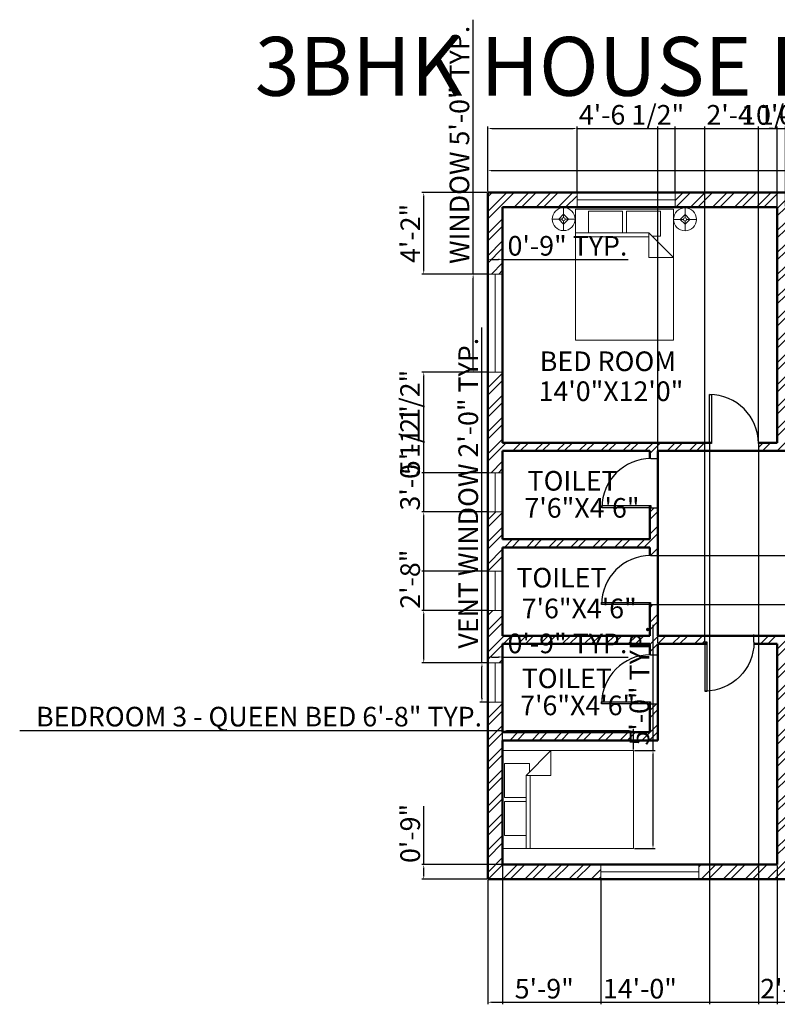
# Model space of a CAD drawing. Units: inches. Extents: x 1954 to 2815, y 1733 to 2371.
# Tile 1 of 4: x 1954 to 2417, y 1769 to 2371. Entities that reach past the tile are written whole.
import ezdxf

# ---------------------------------------------------------------- set-up
doc = ezdxf.new("R2010")
doc.units = ezdxf.units.IN
for name, color, linetype, lineweight in [('A-ANNO-DIMS', 2, 'Continuous', 18), ('A-ANNO-TEXT', 7, 'Continuous', 25), ('A-AREA-IDEN', 7, 'Continuous', 25), ('A-DOOR', 3, 'Continuous', 25), ('A-FURN', 8, 'Continuous', 18), ('A-GLAZ', 4, 'Continuous', 18), ('A-WALL', 7, 'Continuous', 50), ('A-WALL-PATT', 252, 'Continuous', 13)]:
    doc.layers.add(name, color=color, linetype=linetype, lineweight=lineweight)
doc.styles.get("Standard").update_dxf_attribs({"font": 'arial.ttf'})
doc.dimstyles.new('ISO-25', dxfattribs={"dimtxt": 12, "dimasz": 2.5, "dimexe": 1.25, "dimexo": 0.625, "dimtad": 1, "dimdec": 1, "dimlunit": 4, "dimtxsty": 'Standard', "dimcen": 2.5, "dimadec": 0, "dimazin": 0, "dimtfac": 1, "dimtdec": 1, "dimtmove": 0, "dimatfit": 3, "dimfxl": 1, "dimarcsym": 0})

# ---------------------------------------------------------------- blocks, each defined once
blk = doc.blocks.new('*U2')
for p, q in [((0, 0), (0, -6)), ((40, 0), (40, -6))]:
    blk.add_line(p, q)
blk.add_lwpolyline([(0, 0), (0, 40), (1.75, 40), (1.75, 0)], close=True)
blk.add_arc((0, 0), 40, 0, 90)
blk = doc.blocks.new('Bed - Queen')
for p, q in [((0, -80.00003), (0, 0)), ((0, 0), (59.99999, 0)), ((59.99999, 0), (59.99999, -80.00003)), ((7.99999, -1.2), (28.79998, -1.2)), ((7.99999, -14.4), (7.99999, -1.2)), ((28.79998, -1.2), (28.79998, -14.4)), ((31.19999, -1.2), (51.99999, -1.2)), ((31.19999, -14.4), (31.19999, -1.2)), ((51.99999, -1.2), (51.99999, -16.4)), ((0, -14.4), (44.8, -14.4)), ((44.8, -16.8), (0, -16.8)), ((59.99999, -29.6), (44.8, -14.4)), ((44.8, -14.4), (44.8, -29.6)), ((51.99999, -16.4), (46.79936, -16.4)), ((44.8, -29.6), (59.99999, -29.6)), ((59.99999, -80.00003), (0, -80.00003))]:
    blk.add_line(p, q)
blk = doc.blocks.new('Lamp - Table')
for p, q in [((0, 7), (0, 1)), ((-1, 0), (-7, 0)), ((0, 3), (-3, 0)), ((-3, 0), (0, -3)), ((3, 0), (0, 3)), ((0, -3), (3, 0)), ((1, 0), (7, 0)), ((0, -1), (0, -7))]:
    blk.add_line(p, q)
for radius in [7, 1]:
    blk.add_circle((0, 0), radius)
blk = doc.blocks.new('*D10')
at = {"layer": 'A-ANNO-DIMS', "color": 0, "lineweight": -2, "transparency": 16777216}
for p, q in [((2239.88, 2265.61), (2239.88, 2279.68)), ((2242.38, 2278.43), (2717.38, 2278.43)), ((2719.88, 2265.61), (2719.88, 2279.68))]:
    blk.add_line(p, q, dxfattribs=at)
at = {"layer": 'A-ANNO-DIMS', "color": 0, "transparency": 16777216}
for points in [[(2242.38, 2278.85), (2242.38, 2278.01), (2239.88, 2278.43)], [(2717.38, 2278.85), (2717.38, 2278.01), (2719.88, 2278.43)]]:
    blk.add_solid(points, dxfattribs=at)
at = {"layer": 'Defpoints', "color": 0, "transparency": 16777216}
for p in [(2719.88, 2278.43), (2239.88, 2264.98), (2719.88, 2264.98)]:
    blk.add_point(p, dxfattribs=at)
at = {"layer": 'A-ANNO-DIMS', "color": 0, "transparency": 16777216, "insert": (2479.88, 2285.18), "char_height": 12, "attachment_point": 5}
blk.add_mtext("40'", dxfattribs=at)
blk = doc.blocks.new('WIN-60IN')
blk.add_line((4.5, 60), (4.5, 0))
blk.add_lwpolyline([(9, 60), (9, 0), (0, 0), (0, 60)], close=True)
blk = doc.blocks.new('VENT-WIN-24IN')
blk.add_line((4.5, 24), (4.5, 0))
blk.add_lwpolyline([(9, 24), (9, 0), (0, 0), (0, 24)], close=True)
blk = doc.blocks.new('*D14')
at = {"layer": 'A-ANNO-DIMS', "color": 0, "lineweight": -2, "transparency": 16777216}
for p, q in [((2230.88, 2215.14), (2230.88, 2370.74)), ((2239.26, 2215.14), (2229.63, 2215.14)), ((2230.88, 2157.64), (2230.88, 2212.64)), ((2239.26, 2155.14), (2229.63, 2155.14))]:
    blk.add_line(p, q, dxfattribs=at)
at = {"layer": 'A-ANNO-DIMS', "color": 0, "transparency": 16777216}
for points in [[(2230.47, 2212.64), (2231.3, 2212.64), (2230.88, 2215.14)], [(2230.47, 2157.64), (2231.3, 2157.64), (2230.88, 2155.14)]]:
    blk.add_solid(points, dxfattribs=at)
at = {"layer": 'Defpoints', "color": 0, "transparency": 16777216}
for p in [(2230.88, 2215.14), (2239.88, 2215.14), (2239.88, 2155.14)]:
    blk.add_point(p, dxfattribs=at)
at = {"layer": 'A-ANNO-DIMS', "color": 0, "transparency": 16777216, "insert": (2224.05, 2294.19), "char_height": 12, "attachment_point": 5, "rotation": 90}
blk.add_mtext('WINDOW 5\'-0" TYP.', dxfattribs=at)
blk = doc.blocks.new('*D15')
at = {"layer": 'A-ANNO-DIMS', "color": 0, "lineweight": -2, "transparency": 16777216}
for p, q in [((2239.88, 2215.77), (2239.88, 2225.39)), ((2242.38, 2224.14), (2246.38, 2224.14)), ((2248.88, 2215.77), (2248.88, 2225.39)), ((2248.88, 2224.14), (2325.78, 2224.14))]:
    blk.add_line(p, q, dxfattribs=at)
at = {"layer": 'A-ANNO-DIMS', "color": 0, "transparency": 16777216}
for points in [[(2242.38, 2224.56), (2242.38, 2223.73), (2239.88, 2224.14)], [(2246.38, 2224.56), (2246.38, 2223.73), (2248.88, 2224.14)]]:
    blk.add_solid(points, dxfattribs=at)
at = {"layer": 'Defpoints', "color": 0, "transparency": 16777216}
for p in [(2248.88, 2224.14), (2239.88, 2215.14), (2248.88, 2215.14)]:
    blk.add_point(p, dxfattribs=at)
at = {"layer": 'A-ANNO-DIMS', "color": 0, "transparency": 16777216, "insert": (2288.58, 2230.89), "char_height": 12, "attachment_point": 5}
blk.add_mtext('0\'-9" TYP.', dxfattribs=at)
blk = doc.blocks.new('*D18')
at = {"layer": 'A-ANNO-DIMS', "color": 0, "lineweight": -2, "transparency": 16777216}
for p, q in [((2248.88, 1935.73), (1953.62, 1935.73)), ((2248.88, 1924.36), (2248.88, 1936.98)), ((2326.38, 1935.73), (2251.38, 1935.73)), ((2328.88, 1924.36), (2328.88, 1936.98))]:
    blk.add_line(p, q, dxfattribs=at)
at = {"layer": 'A-ANNO-DIMS', "color": 0, "transparency": 16777216}
for points in [[(2251.38, 1936.15), (2251.38, 1935.32), (2248.88, 1935.73)], [(2326.38, 1936.15), (2326.38, 1935.32), (2328.88, 1935.73)]]:
    blk.add_solid(points, dxfattribs=at)
at = {"layer": 'Defpoints', "color": 0, "transparency": 16777216}
for p in [(2248.88, 1935.73), (2248.88, 1923.73), (2328.88, 1923.73)]:
    blk.add_point(p, dxfattribs=at)
at = {"layer": 'A-ANNO-DIMS', "color": 0, "transparency": 16777216, "insert": (2100, 1942.93), "char_height": 12, "attachment_point": 5}
blk.add_mtext('BEDROOM 3 - QUEEN BED 6\'-8" TYP.', dxfattribs=at)
blk = doc.blocks.new('*D19')
at = {"layer": 'A-ANNO-DIMS', "color": 0, "lineweight": -2, "transparency": 16777216}
for p, q in [((2340.88, 1923.73), (2340.88, 2000.63)), ((2329.51, 1923.73), (2342.13, 1923.73)), ((2340.88, 1866.23), (2340.88, 1921.23)), ((2329.51, 1863.73), (2342.13, 1863.73))]:
    blk.add_line(p, q, dxfattribs=at)
at = {"layer": 'A-ANNO-DIMS', "color": 0, "transparency": 16777216}
for points in [[(2340.47, 1921.23), (2341.3, 1921.23), (2340.88, 1923.73)], [(2340.47, 1866.23), (2341.3, 1866.23), (2340.88, 1863.73)]]:
    blk.add_solid(points, dxfattribs=at)
at = {"layer": 'Defpoints', "color": 0, "transparency": 16777216}
for p in [(2328.88, 1923.73), (2340.88, 1923.73), (2328.88, 1863.73)]:
    blk.add_point(p, dxfattribs=at)
at = {"layer": 'A-ANNO-DIMS', "color": 0, "transparency": 16777216, "insert": (2334.13, 1963.43), "char_height": 12, "attachment_point": 5, "rotation": 90}
blk.add_mtext('5\'-0" TYP.', dxfattribs=at)
blk = doc.blocks.new('*D20')
at = {"layer": 'A-ANNO-DIMS', "color": 0, "lineweight": -2, "transparency": 16777216}
for p, q in [((2236.28, 1977.35), (2236.28, 2182.45)), ((2239.26, 1977.35), (2235.03, 1977.35)), ((2236.28, 1955.85), (2236.28, 1974.85)), ((2239.26, 1953.35), (2235.03, 1953.35))]:
    blk.add_line(p, q, dxfattribs=at)
at = {"layer": 'A-ANNO-DIMS', "color": 0, "transparency": 16777216}
for points in [[(2235.87, 1974.85), (2236.7, 1974.85), (2236.28, 1977.35)], [(2235.87, 1955.85), (2236.7, 1955.85), (2236.28, 1953.35)]]:
    blk.add_solid(points, dxfattribs=at)
at = {"layer": 'Defpoints', "color": 0, "transparency": 16777216}
for p in [(2236.28, 1977.35), (2239.88, 1977.35), (2239.88, 1953.35)]:
    blk.add_point(p, dxfattribs=at)
at = {"layer": 'A-ANNO-DIMS', "color": 0, "transparency": 16777216, "insert": (2229.45, 2081.15), "char_height": 12, "attachment_point": 5, "rotation": 90}
blk.add_mtext('VENT WINDOW 2\'-0" TYP.', dxfattribs=at)
blk = doc.blocks.new('*D21')
at = {"layer": 'A-ANNO-DIMS', "color": 0, "lineweight": -2, "transparency": 16777216}
for p, q in [((2239.88, 1977.98), (2239.88, 1982.2)), ((2248.88, 1977.98), (2248.88, 1982.2)), ((2242.38, 1980.95), (2246.38, 1980.95)), ((2248.88, 1980.95), (2325.78, 1980.95))]:
    blk.add_line(p, q, dxfattribs=at)
at = {"layer": 'A-ANNO-DIMS', "color": 0, "transparency": 16777216}
for points in [[(2242.38, 1981.37), (2242.38, 1980.54), (2239.88, 1980.95)], [(2246.38, 1981.37), (2246.38, 1980.54), (2248.88, 1980.95)]]:
    blk.add_solid(points, dxfattribs=at)
at = {"layer": 'Defpoints', "color": 0, "transparency": 16777216}
for p in [(2239.88, 1977.35), (2248.88, 1980.95), (2248.88, 1977.35)]:
    blk.add_point(p, dxfattribs=at)
at = {"layer": 'A-ANNO-DIMS', "color": 0, "transparency": 16777216, "insert": (2288.58, 1987.71), "char_height": 12, "attachment_point": 5}
blk.add_mtext('0\'-9" TYP.', dxfattribs=at)
blk = doc.blocks.new('*D30')
at = {"layer": 'A-ANNO-DIMS', "color": 0, "lineweight": -2, "transparency": 16777216}
for p, q in [((2248.88, 1853.36), (2248.88, 1768.53)), ((2416.88, 1853.36), (2416.88, 1768.53)), ((2251.38, 1769.78), (2414.38, 1769.78))]:
    blk.add_line(p, q, dxfattribs=at)
at = {"layer": 'A-ANNO-DIMS', "color": 0, "transparency": 16777216}
for points in [[(2251.38, 1770.2), (2251.38, 1769.37), (2248.88, 1769.78)], [(2414.38, 1770.2), (2414.38, 1769.37), (2416.88, 1769.78)]]:
    blk.add_solid(points, dxfattribs=at)
at = {"layer": 'Defpoints', "color": 0, "transparency": 16777216}
for p in [(2248.88, 1853.98), (2416.88, 1853.98), (2416.88, 1769.78)]:
    blk.add_point(p, dxfattribs=at)
at = {"layer": 'A-ANNO-DIMS', "color": 0, "transparency": 16777216, "insert": (2332.88, 1776.53), "char_height": 12, "attachment_point": 5}
blk.add_mtext('14\'-0"', dxfattribs=at)
blk = doc.blocks.new('*D36')
at = {"layer": 'A-ANNO-DIMS', "color": 0, "lineweight": -2, "transparency": 16777216}
for p, q in [((2200.68, 1853.98), (2200.68, 1889.63)), ((2248.26, 1853.98), (2199.43, 1853.98)), ((2200.68, 1847.48), (2200.68, 1851.48)), ((2239.26, 1844.98), (2199.43, 1844.98))]:
    blk.add_line(p, q, dxfattribs=at)
at = {"layer": 'A-ANNO-DIMS', "color": 0, "transparency": 16777216}
for points in [[(2200.27, 1851.48), (2201.1, 1851.48), (2200.68, 1853.98)], [(2200.27, 1847.48), (2201.1, 1847.48), (2200.68, 1844.98)]]:
    blk.add_solid(points, dxfattribs=at)
at = {"layer": 'Defpoints', "color": 0, "transparency": 16777216}
for p in [(2200.68, 1853.98), (2248.88, 1853.98), (2239.88, 1844.98)]:
    blk.add_point(p, dxfattribs=at)
at = {"layer": 'A-ANNO-DIMS', "color": 0, "transparency": 16777216, "insert": (2193.93, 1873.06), "char_height": 12, "attachment_point": 5, "rotation": 90}
blk.add_mtext('0\'-9"', dxfattribs=at)
blk = doc.blocks.new('*D37')
at = {"layer": 'A-ANNO-DIMS', "color": 0, "lineweight": -2, "transparency": 16777216}
for p, q in [((2414.38, 2304.18), (2411.88, 2304.18)), ((2416.88, 2256.61), (2416.88, 2305.43)), ((2416.88, 2304.18), (2421.88, 2304.18)), ((2421.88, 2256.61), (2421.88, 2305.43)), ((2424.38, 2304.18), (2460.03, 2304.18))]:
    blk.add_line(p, q, dxfattribs=at)
at = {"layer": 'A-ANNO-DIMS', "color": 0, "transparency": 16777216}
for points in [[(2414.38, 2304.6), (2414.38, 2303.77), (2416.88, 2304.18)], [(2424.38, 2304.6), (2424.38, 2303.77), (2421.88, 2304.18)]]:
    blk.add_solid(points, dxfattribs=at)
at = {"layer": 'Defpoints', "color": 0, "transparency": 16777216}
for p in [(2421.88, 2304.18), (2416.88, 2255.98), (2421.88, 2255.98)]:
    blk.add_point(p, dxfattribs=at)
at = {"layer": 'A-ANNO-DIMS', "color": 0, "transparency": 16777216, "insert": (2443.46, 2310.93), "char_height": 12, "attachment_point": 5}
blk.add_mtext('0\'-5"', dxfattribs=at)
blk = doc.blocks.new('*D38')
at = {"layer": 'A-ANNO-DIMS', "color": 0, "lineweight": -2, "transparency": 16777216}
for p, q in [((2239.88, 2265.61), (2239.88, 2305.43)), ((2242.38, 2304.18), (2291.96, 2304.18)), ((2294.46, 2265.61), (2294.46, 2305.43)), ((2294.46, 2304.18), (2358.55, 2304.18))]:
    blk.add_line(p, q, dxfattribs=at)
at = {"layer": 'A-ANNO-DIMS', "color": 0, "transparency": 16777216}
for points in [[(2242.38, 2304.6), (2242.38, 2303.77), (2239.88, 2304.18)], [(2291.96, 2304.6), (2291.96, 2303.77), (2294.46, 2304.18)]]:
    blk.add_solid(points, dxfattribs=at)
at = {"layer": 'Defpoints', "color": 0, "transparency": 16777216}
for p in [(2294.46, 2304.18), (2239.88, 2264.98), (2294.46, 2264.98)]:
    blk.add_point(p, dxfattribs=at)
at = {"layer": 'A-ANNO-DIMS', "color": 0, "transparency": 16777216, "insert": (2327.76, 2311.01), "char_height": 12, "attachment_point": 5}
blk.add_mtext('4\'-6 1/2"', dxfattribs=at)
blk = doc.blocks.new('*D39')
at = {"layer": 'A-ANNO-DIMS', "color": 0, "lineweight": -2, "transparency": 16777216}
for p, q in [((2354.46, 2265.61), (2354.46, 2305.43)), ((2356.96, 2304.18), (2477.93, 2304.18)), ((2480.43, 2265.61), (2480.43, 2305.43))]:
    blk.add_line(p, q, dxfattribs=at)
at = {"layer": 'A-ANNO-DIMS', "color": 0, "transparency": 16777216}
for points in [[(2356.96, 2304.6), (2356.96, 2303.77), (2354.46, 2304.18)], [(2477.93, 2304.6), (2477.93, 2303.77), (2480.43, 2304.18)]]:
    blk.add_solid(points, dxfattribs=at)
at = {"layer": 'Defpoints', "color": 0, "transparency": 16777216}
for p in [(2480.43, 2304.18), (2354.46, 2264.98), (2480.43, 2264.98)]:
    blk.add_point(p, dxfattribs=at)
at = {"layer": 'A-ANNO-DIMS', "color": 0, "transparency": 16777216, "insert": (2417.44, 2310.93), "char_height": 12, "attachment_point": 5}
blk.add_mtext('10\'-6"', dxfattribs=at)
blk = doc.blocks.new('*D40')
at = {"layer": 'A-ANNO-DIMS', "color": 0, "lineweight": -2, "transparency": 16777216}
for p, q in [((2239.88, 1844.36), (2239.88, 1768.53)), ((2308.9, 1844.36), (2308.9, 1768.53)), ((2242.38, 1769.78), (2306.4, 1769.78))]:
    blk.add_line(p, q, dxfattribs=at)
at = {"layer": 'A-ANNO-DIMS', "color": 0, "transparency": 16777216}
for points in [[(2242.38, 1770.2), (2242.38, 1769.37), (2239.88, 1769.78)], [(2306.4, 1770.2), (2306.4, 1769.37), (2308.9, 1769.78)]]:
    blk.add_solid(points, dxfattribs=at)
at = {"layer": 'Defpoints', "color": 0, "transparency": 16777216}
for p in [(2239.88, 1844.98), (2308.9, 1844.98), (2308.9, 1769.78)]:
    blk.add_point(p, dxfattribs=at)
at = {"layer": 'A-ANNO-DIMS', "color": 0, "transparency": 16777216, "insert": (2274.39, 1776.53), "char_height": 12, "attachment_point": 5}
blk.add_mtext('5\'-9"', dxfattribs=at)
blk = doc.blocks.new('*D41')
at = {"layer": 'A-ANNO-DIMS', "color": 0, "lineweight": -2, "transparency": 16777216}
for p, q in [((2239.26, 2264.98), (2199.43, 2264.98)), ((2200.68, 2217.64), (2200.68, 2262.48)), ((2239.26, 2215.14), (2199.43, 2215.14))]:
    blk.add_line(p, q, dxfattribs=at)
at = {"layer": 'A-ANNO-DIMS', "color": 0, "transparency": 16777216}
for points in [[(2200.27, 2262.48), (2201.1, 2262.48), (2200.68, 2264.98)], [(2200.27, 2217.64), (2201.1, 2217.64), (2200.68, 2215.14)]]:
    blk.add_solid(points, dxfattribs=at)
at = {"layer": 'Defpoints', "color": 0, "transparency": 16777216}
for p in [(2200.68, 2264.98), (2239.88, 2264.98), (2239.88, 2215.14)]:
    blk.add_point(p, dxfattribs=at)
at = {"layer": 'A-ANNO-DIMS', "color": 0, "transparency": 16777216, "insert": (2194.03, 2240.06), "char_height": 12, "attachment_point": 5, "rotation": 90}
blk.add_mtext('4\'-2"', dxfattribs=at)
blk = doc.blocks.new('*D42')
at = {"layer": 'A-ANNO-DIMS', "color": 0, "lineweight": -2, "transparency": 16777216}
for p, q in [((2239.26, 2155.14), (2199.43, 2155.14)), ((2200.68, 2096.18), (2200.68, 2152.64)), ((2239.26, 2093.68), (2199.43, 2093.68))]:
    blk.add_line(p, q, dxfattribs=at)
at = {"layer": 'A-ANNO-DIMS', "color": 0, "transparency": 16777216}
for points in [[(2200.27, 2152.64), (2201.1, 2152.64), (2200.68, 2155.14)], [(2200.27, 2096.18), (2201.1, 2096.18), (2200.68, 2093.68)]]:
    blk.add_solid(points, dxfattribs=at)
at = {"layer": 'Defpoints', "color": 0, "transparency": 16777216}
for p in [(2200.68, 2155.14), (2239.88, 2155.14), (2239.88, 2093.68)]:
    blk.add_point(p, dxfattribs=at)
at = {"layer": 'A-ANNO-DIMS', "color": 0, "transparency": 16777216, "insert": (2193.85, 2124.41), "char_height": 12, "attachment_point": 5, "rotation": 90}
blk.add_mtext('5\'-1 1/2"', dxfattribs=at)
blk = doc.blocks.new('*D43')
at = {"layer": 'A-ANNO-DIMS', "color": 0, "lineweight": -2, "transparency": 16777216}
for p, q in [((2200.68, 2069.68), (2200.68, 2133.29)), ((2239.26, 2069.68), (2199.43, 2069.68)), ((2200.68, 2035.9), (2200.68, 2067.18)), ((2239.26, 2033.4), (2199.43, 2033.4))]:
    blk.add_line(p, q, dxfattribs=at)
at = {"layer": 'A-ANNO-DIMS', "color": 0, "transparency": 16777216}
for points in [[(2200.27, 2067.18), (2201.1, 2067.18), (2200.68, 2069.68)], [(2200.27, 2035.9), (2201.1, 2035.9), (2200.68, 2033.4)]]:
    blk.add_solid(points, dxfattribs=at)
at = {"layer": 'Defpoints', "color": 0, "transparency": 16777216}
for p in [(2200.68, 2069.68), (2239.88, 2069.68), (2239.88, 2033.4)]:
    blk.add_point(p, dxfattribs=at)
at = {"layer": 'A-ANNO-DIMS', "color": 0, "transparency": 16777216, "insert": (2193.85, 2102.74), "char_height": 12, "attachment_point": 5, "rotation": 90}
blk.add_mtext('3\'-0 1/2"', dxfattribs=at)
blk = doc.blocks.new('*D44')
at = {"layer": 'A-ANNO-DIMS', "color": 0, "lineweight": -2, "transparency": 16777216}
for p, q in [((2200.68, 2009.4), (2200.68, 2045.25)), ((2239.26, 2009.4), (2199.43, 2009.4)), ((2200.68, 1979.85), (2200.68, 2006.9)), ((2239.26, 1977.35), (2199.43, 1977.35))]:
    blk.add_line(p, q, dxfattribs=at)
at = {"layer": 'A-ANNO-DIMS', "color": 0, "transparency": 16777216}
for points in [[(2200.27, 2006.9), (2201.1, 2006.9), (2200.68, 2009.4)], [(2200.27, 1979.85), (2201.1, 1979.85), (2200.68, 1977.35)]]:
    blk.add_solid(points, dxfattribs=at)
at = {"layer": 'Defpoints', "color": 0, "transparency": 16777216}
for p in [(2200.68, 2009.4), (2239.88, 2009.4), (2239.88, 1977.35)]:
    blk.add_point(p, dxfattribs=at)
at = {"layer": 'A-ANNO-DIMS', "color": 0, "transparency": 16777216, "insert": (2193.93, 2028.57), "char_height": 12, "attachment_point": 5, "rotation": 90}
blk.add_mtext('2\'-8"', dxfattribs=at)
blk = doc.blocks.new('*D47')
at = {"layer": 'A-ANNO-DIMS', "color": 0, "lineweight": -2, "transparency": 16777216}
for p, q in [((2375.36, 2106.36), (2375.36, 1768.53)), ((2405.36, 2106.36), (2405.36, 1768.53)), ((2377.86, 1769.78), (2402.86, 1769.78)), ((2405.36, 1769.78), (2441.21, 1769.78))]:
    blk.add_line(p, q, dxfattribs=at)
at = {"layer": 'A-ANNO-DIMS', "color": 0, "transparency": 16777216}
for points in [[(2377.86, 1770.2), (2377.86, 1769.37), (2375.36, 1769.78)], [(2402.86, 1770.2), (2402.86, 1769.37), (2405.36, 1769.78)]]:
    blk.add_solid(points, dxfattribs=at)
at = {"layer": 'Defpoints', "color": 0, "transparency": 16777216}
for p in [(2375.36, 2106.98), (2405.36, 2106.98), (2405.36, 1769.78)]:
    blk.add_point(p, dxfattribs=at)
at = {"layer": 'A-ANNO-DIMS', "color": 0, "transparency": 16777216, "insert": (2424.53, 1776.53), "char_height": 12, "attachment_point": 5}
blk.add_mtext('2\'-6"', dxfattribs=at)
blk = doc.blocks.new('*D48')
at = {"layer": 'A-ANNO-DIMS', "color": 0, "lineweight": -2, "transparency": 16777216}
for p, q in [((2405.35, 2112.61), (2405.35, 2305.43)), ((2407.85, 2304.18), (2414.38, 2304.18)), ((2416.88, 2112.61), (2416.88, 2305.43)), ((2416.88, 2304.18), (2489.82, 2304.18))]:
    blk.add_line(p, q, dxfattribs=at)
at = {"layer": 'A-ANNO-DIMS', "color": 0, "transparency": 16777216}
for points in [[(2407.85, 2304.6), (2407.85, 2303.77), (2405.35, 2304.18)], [(2414.38, 2304.6), (2414.38, 2303.77), (2416.88, 2304.18)]]:
    blk.add_solid(points, dxfattribs=at)
at = {"layer": 'Defpoints', "color": 0, "transparency": 16777216}
for p in [(2416.88, 2304.18), (2405.35, 2111.98), (2416.88, 2111.98)]:
    blk.add_point(p, dxfattribs=at)
at = {"layer": 'A-ANNO-DIMS', "color": 0, "transparency": 16777216, "insert": (2454.6, 2311.01), "char_height": 12, "attachment_point": 5}
blk.add_mtext('0\'-11 1/2"', dxfattribs=at)
blk = doc.blocks.new('*D52')
at = {"layer": 'A-ANNO-DIMS', "color": 0, "lineweight": -2, "transparency": 16777216}
for p, q in [((2759.08, 2043), (2759.08, 2078.85)), ((2344.56, 2043), (2760.33, 2043)), ((2759.08, 2015.5), (2759.08, 2040.5)), ((2344.56, 2013), (2760.33, 2013))]:
    blk.add_line(p, q, dxfattribs=at)
at = {"layer": 'A-ANNO-DIMS', "color": 0, "transparency": 16777216}
for points in [[(2758.67, 2040.5), (2759.5, 2040.5), (2759.08, 2043)], [(2758.67, 2015.5), (2759.5, 2015.5), (2759.08, 2013)]]:
    blk.add_solid(points, dxfattribs=at)
at = {"layer": 'Defpoints', "color": 0, "transparency": 16777216}
for p in [(2343.94, 2043), (2759.08, 2043), (2343.94, 2013)]:
    blk.add_point(p, dxfattribs=at)
at = {"layer": 'A-ANNO-DIMS', "color": 0, "transparency": 16777216, "insert": (2752.33, 2062.18), "char_height": 12, "attachment_point": 5, "rotation": 90}
blk.add_mtext('2\'-6"', dxfattribs=at)
blk = doc.blocks.new('*D55')
at = {"layer": 'A-ANNO-DIMS', "color": 0, "lineweight": -2, "transparency": 16777216}
for p, q in [((2343.88, 1989.61), (2343.88, 2305.43)), ((2346.38, 2304.18), (2370.09, 2304.18)), ((2372.59, 1990.74), (2372.59, 2305.43)), ((2372.59, 2304.18), (2436.4, 2304.18))]:
    blk.add_line(p, q, dxfattribs=at)
at = {"layer": 'A-ANNO-DIMS', "color": 0, "transparency": 16777216}
for points in [[(2346.38, 2304.6), (2346.38, 2303.77), (2343.88, 2304.18)], [(2370.09, 2304.6), (2370.09, 2303.77), (2372.59, 2304.18)]]:
    blk.add_solid(points, dxfattribs=at)
at = {"layer": 'Defpoints', "color": 0, "transparency": 16777216}
for p in [(2372.59, 2304.18), (2343.88, 1988.98), (2372.59, 1990.12)]:
    blk.add_point(p, dxfattribs=at)
at = {"layer": 'A-ANNO-DIMS', "color": 0, "transparency": 16777216, "insert": (2405.75, 2311.01), "char_height": 12, "attachment_point": 5}
blk.add_mtext('2\'-4 1/2"', dxfattribs=at)

msp = doc.modelspace()

# ---------------------------------------------------------------- hatches: boundary and pattern name
at = {"layer": 'A-WALL-PATT'}
h = msp.add_hatch(dxfattribs=at)
h.set_pattern_fill('ANSI32', color=256)
h.paths.add_polyline_path([(2294.46, 2264.98), (2239.88, 2264.98), (2239.88, 2215.14), (2248.88, 2215.14), (2248.88, 2255.98), (2294.46, 2255.98)])
h = msp.add_hatch(dxfattribs=at)
h.set_pattern_fill('ANSI32', color=256)
h.paths.add_polyline_path([(2480.43, 2264.98), (2354.46, 2264.98), (2354.46, 2255.98), (2416.88, 2255.98), (2416.88, 2111.98), (2405.35, 2111.98, -0.004167), (2405.36, 2111.48), (2405.36, 2106.98), (2487.77, 2106.98), (2487.77, 2111.48), (2487.77, 2111.98), (2421.88, 2111.98), (2421.88, 2255.98), (2480.43, 2255.98)])
h.paths.add_polyline_path([(2719.88, 2264.98), (2540.43, 2264.98), (2540.43, 2255.98), (2589.88, 2255.98), (2589.88, 2111.98), (2517.77, 2111.98, -0.004167), (2517.77, 2111.48), (2517.77, 2106.98), (2631.3, 2106.98), (2631.3, 2111.98), (2594.88, 2111.98), (2594.88, 2255.98), (2710.88, 2255.98), (2710.88, 2213), (2719.88, 2213)])
h = msp.add_hatch(dxfattribs=at)
h.set_pattern_fill('ANSI32', color=256)
h.paths.add_polyline_path([(2375.36, 2111.48), (2375.36, 2111.98), (2248.88, 2111.98), (2248.88, 2155.14), (2239.88, 2155.14), (2239.88, 2093.68), (2248.88, 2093.68), (2248.88, 2106.98), (2338.88, 2106.98), (2338.88, 2102.27, -0.006284), (2339.64, 2102.28), (2343.88, 2102.28), (2343.88, 2106.98), (2375.36, 2106.98)])
h.paths.add_polyline_path([(2343.88, 2052.98), (2343.88, 2072.28), (2339.64, 2072.28), (2338.88, 2072.28), (2338.88, 2052.98), (2248.88, 2052.98), (2248.88, 2069.68), (2239.88, 2069.68), (2239.88, 2033.4), (2248.88, 2033.4), (2248.88, 2047.98), (2338.88, 2047.98), (2338.88, 2042.99, -0.004601), (2339.44, 2043), (2343.88, 2043)])
h = msp.add_hatch(dxfattribs=at)
h.set_pattern_fill('ANSI32', color=256)
h.paths.add_polyline_path([(2372.59, 1993.98), (2343.88, 1993.98), (2343.88, 2013), (2339.44, 2013), (2338.88, 2013), (2338.88, 1993.98), (2248.88, 1993.98), (2248.88, 2009.4), (2239.88, 2009.4), (2239.88, 1977.35), (2248.88, 1977.35), (2248.88, 1988.98), (2338.88, 1988.98), (2338.88, 1982.3, -0.004167), (2339.38, 1982.31), (2343.88, 1982.31), (2343.88, 1988.98), (2372.59, 1988.98), (2372.59, 1990.12)])
h = msp.add_hatch(dxfattribs=at)
h.set_pattern_fill('ANSI32', color=256)
h.paths.add_polyline_path([(2585.41, 1844.98), (2585.41, 1849.48, -0.03766), (2585.75, 1853.98), (2486.88, 1853.98), (2486.88, 1942.98), (2471.49, 1942.98), (2471.49, 1937.98), (2481.88, 1937.98), (2481.88, 1853.98), (2421.88, 1853.98), (2421.88, 1937.98), (2435.43, 1937.98), (2435.43, 1942.98), (2421.88, 1942.98), (2421.88, 1993.98), (2402.59, 1993.98), (2402.59, 1990.12, -0.009455), (2402.57, 1988.98), (2416.88, 1988.98), (2416.88, 1853.98), (2368.9, 1853.98), (2368.9, 1844.98)])
h.paths.add_polyline_path([(2308.9, 1844.98), (2308.9, 1853.98), (2248.88, 1853.98), (2248.88, 1929.98), (2343.88, 1929.98), (2343.88, 1952.31), (2339.38, 1952.31), (2338.88, 1952.31), (2338.88, 1934.98), (2248.88, 1934.98), (2248.88, 1953.35), (2239.88, 1953.35), (2239.88, 1844.98)])

# ---------------------------------------------------------------- linework, layer by layer
at = {"layer": 'A-WALL'}
for p, q in [((2239.88, 2264.98), (2719.88, 2264.98)), ((2239.88, 1844.98), (2239.88, 2264.98)), ((2248.88, 2255.98), (2416.88, 2255.98)), ((2248.88, 2111.98), (2248.88, 2255.98)), ((2416.88, 2111.98), (2416.88, 2255.98)), ((2248.88, 2111.98), (2376.67, 2111.98)), ((2405.35, 2111.98), (2416.88, 2111.98)), ((2248.88, 2106.98), (2338.88, 2106.98)), ((2248.88, 2052.98), (2248.88, 2106.98)), ((2338.88, 2102.27), (2338.88, 2106.98)), ((2343.88, 2052.98), (2343.88, 2106.98)), ((2343.88, 2106.98), (2631.3, 2106.98)), ((2338.88, 2052.98), (2338.88, 2073.6)), ((2248.88, 2052.98), (2338.88, 2052.98)), ((2248.88, 2047.98), (2338.88, 2047.98)), ((2248.88, 1993.98), (2248.88, 2047.98)), ((2338.88, 2042.99), (2338.88, 2047.98)), ((2343.88, 1993.98), (2343.88, 2052.98)), ((2338.88, 1993.98), (2338.88, 2014.31)), ((2248.88, 1993.98), (2338.88, 1993.98)), ((2343.88, 1993.98), (2421.88, 1993.98)), ((2248.88, 1988.98), (2338.88, 1988.98)), ((2248.88, 1934.98), (2248.88, 1988.98)), ((2338.88, 1982.3), (2338.88, 1988.98)), ((2343.88, 1929.98), (2343.88, 1988.98)), ((2343.88, 1988.98), (2373.9, 1988.98)), ((2402.57, 1988.98), (2416.88, 1988.98)), ((2416.88, 1853.98), (2416.88, 1988.98)), ((2338.88, 1934.98), (2338.88, 1953.62)), ((2248.88, 1934.98), (2338.88, 1934.98)), ((2248.88, 1853.98), (2248.88, 1929.98)), ((2248.88, 1929.98), (2343.88, 1929.98)), ((2416.88, 1853.98), (2248.88, 1853.98)), ((2719.88, 1844.98), (2239.88, 1844.98))]:
    msp.add_line(p, q, dxfattribs=at)

# ---------------------------------------------------------------- block references
at = {"layer": 'A-DOOR', "xscale": 0.75, "yscale": 0.75, "zscale": 0.75}
msp.add_blockref('*U2', (2375.36, 2111.48), dxfattribs=at)
at = {"layer": 'A-DOOR', "yscale": 0.75, "zscale": 0.75}
for p, xscale, rotation in [((2339.64, 2072.28), 0.75, 90), ((2339.44, 2013), 0.75, 90), ((2372.59, 1990.12), -0.75, 180), ((2339.38, 1952.31), 0.75, 90)]:
    msp.add_blockref('*U2', p, dxfattribs=dict(at, xscale=xscale, rotation=rotation))
at = {"layer": 'A-FURN'}
for name, p in [('Lamp - Table', (2286.23, 2248.74)), ('Bed - Queen', (2293.46, 2254.81)), ('Lamp - Table', (2360.46, 2248.61))]:
    msp.add_blockref(name, p, dxfattribs=at)
at = {"layer": 'A-FURN', "rotation": 89.99999999999999}
msp.add_blockref('Bed - Queen', (2248.88, 1863.73), dxfattribs=at)
at = {"layer": 'A-GLAZ'}
for p, rotation in [((2354.46, 2255.98), 90.00000000000011), ((2368.9, 1844.98), 90.00000000000003)]:
    msp.add_blockref('WIN-60IN', p, dxfattribs=dict(at, rotation=rotation))
for name, p in [('WIN-60IN', (2239.88, 2155.14)), ('VENT-WIN-24IN', (2239.88, 2069.68)), ('VENT-WIN-24IN', (2239.88, 2009.4)), ('VENT-WIN-24IN', (2239.88, 1953.35))]:
    msp.add_blockref(name, p, dxfattribs=at)

# ---------------------------------------------------------------- texts
at = {"layer": 'A-ANNO-TEXT'}
msp.add_text('3BHK HOUSE PLAN 40\'0"X35\'0"', height=36, dxfattribs=at).set_placement((2097.45, 2324.21))
at = {"layer": 'A-AREA-IDEN'}
for s, p in [('BED ROOM', (2271.65, 2155.83)), ('14\'0"X12\'0"', (2270.92, 2137.51)), ('TOILET', (2264.17, 2082.73)), ('7\'6"X4\'6"', (2262.28, 2066.16)), ('TOILET', (2257.33, 2023.48)), ('7\'6"X4\'6"', (2260.59, 2004.64)), ('TOILET', (2260.59, 1961.9)), ('7\'6"X4\'6"', (2259.67, 1945.35))]:
    msp.add_text(s, height=12, dxfattribs=at).set_placement(p)

# ---------------------------------------------------------------- dimensions: what is measured, and where the dimension line sits
at = {"layer": 'A-ANNO-DIMS'}
for base, p1, p2, angle, text, picture, middle in [((2230.88, 2215.14), (2239.88, 2155.14), (2239.88, 2215.14), 90, 'WINDOW <> TYP.', '*D14', (2224.05, 2294.19)), ((2236.28, 1977.35), (2239.88, 1953.35), (2239.88, 1977.35), 90, 'VENT WINDOW <> TYP.', '*D20', (2229.45, 2081.15)), ((2248.88, 1935.73), (2328.88, 1923.73), (2248.88, 1923.73), 180, 'BEDROOM 3 - QUEEN BED <> TYP.', '*D18', (2100, 1942.93)), ((2340.88, 1923.73), (2328.88, 1863.73), (2328.88, 1923.73), 90, '<> TYP.', '*D19', (2334.13, 1963.43))]:
    dim = msp.add_linear_dim(base=base, p1=p1, p2=p2, angle=angle, text=text, dimstyle='ISO-25', override={"dimdec": 1, "dimlfac": 1, "dimrnd": 0, "dimzin": 1, "dimdsep": 46, "dimlunit": 4, "dimfrac": 2}, dxfattribs=at)
    dim.commit()
    dim.dimension.update_dxf_attribs({"geometry": picture, "text_midpoint": middle})
for base, p1, p2, override, picture, middle in [((2294.46, 2304.18), (2239.88, 2264.98), (2294.46, 2264.98), {"dimdec": 1, "dimlfac": 1, "dimrnd": 0, "dimzin": 1, "dimdsep": 46, "dimlunit": 4, "dimfrac": 2}, '*D38', (2327.76, 2311.01)), ((2372.59, 2304.18), (2343.88, 1988.98), (2372.59, 1990.12), {"dimdec": 1, "dimlfac": 1, "dimrnd": 0, "dimzin": 1, "dimdsep": 46, "dimlunit": 4, "dimfrac": 2}, '*D55', (2405.75, 2311.01)), ((2416.88, 2304.18), (2405.35, 2111.98), (2416.88, 2111.98), {"dimdec": 1, "dimlfac": 1, "dimrnd": 0, "dimzin": 1, "dimdsep": 46, "dimlunit": 4, "dimfrac": 2}, '*D48', (2454.6, 2311.01)), ((2480.43, 2304.18), (2354.46, 2264.98), (2480.43, 2264.98), {"dimdec": 1, "dimlfac": 1, "dimrnd": 0, "dimzin": 1, "dimdsep": 46, "dimlunit": 4, "dimfrac": 2}, '*D39', (2417.44, 2310.93)), ((2421.88, 2304.18), (2416.88, 2255.98), (2421.88, 2255.98), {"dimdec": 1, "dimlfac": 1, "dimrnd": 0, "dimzin": 1, "dimdsep": 46, "dimlunit": 4, "dimfrac": 2}, '*D37', (2443.46, 2310.93)), ((2719.88, 2278.43), (2239.88, 2264.98), (2719.88, 2264.98), {"dimclrd": 0, "dimclre": 0, "dimclrt": 0}, '*D10', (2479.88, 2285.18)), ((2405.36, 1769.78), (2375.36, 2106.98), (2405.36, 2106.98), {"dimdec": 1, "dimlfac": 1, "dimrnd": 0, "dimzin": 1, "dimdsep": 46, "dimlunit": 4, "dimfrac": 2}, '*D47', (2424.53, 1776.53)), ((2416.88, 1769.78), (2248.88, 1853.98), (2416.88, 1853.98), {"dimdec": 1, "dimlfac": 1, "dimrnd": 0, "dimzin": 1, "dimdsep": 46, "dimlunit": 4, "dimfrac": 2}, '*D30', (2332.88, 1776.53)), ((2308.9, 1769.78), (2239.88, 1844.98), (2308.9, 1844.98), {"dimdec": 1, "dimlfac": 1, "dimrnd": 0, "dimzin": 1, "dimdsep": 46, "dimlunit": 4, "dimfrac": 2}, '*D40', (2274.39, 1776.53))]:
    dim = msp.add_linear_dim(base=base, p1=p1, p2=p2, dimstyle='ISO-25', override=override, dxfattribs=at)
    dim.commit()
    dim.dimension.update_dxf_attribs({"geometry": picture, "text_midpoint": middle})
for base, p1, p2, picture, middle in [((2200.68, 2264.98), (2239.88, 2215.14), (2239.88, 2264.98), '*D41', (2194.03, 2240.06)), ((2200.68, 2155.14), (2239.88, 2093.68), (2239.88, 2155.14), '*D42', (2193.85, 2124.41)), ((2200.68, 2069.68), (2239.88, 2033.4), (2239.88, 2069.68), '*D43', (2193.85, 2102.74)), ((2759.08, 2043), (2343.94, 2013), (2343.94, 2043), '*D52', (2752.33, 2062.18)), ((2200.6844, 2009.3974), (2239.8844, 1977.3533), (2239.8844, 2009.3974), '*D44', (2193.9325, 2028.5743)), ((2200.68, 1853.98), (2239.88, 1844.98), (2248.88, 1853.98), '*D36', (2193.93, 1873.06))]:
    dim = msp.add_linear_dim(base=base, p1=p1, p2=p2, angle=90, dimstyle='ISO-25', override={"dimdec": 1, "dimlfac": 1, "dimrnd": 0, "dimzin": 1, "dimdsep": 46, "dimlunit": 4, "dimfrac": 2}, dxfattribs=at)
    dim.commit()
    dim.dimension.update_dxf_attribs({"geometry": picture, "text_midpoint": middle})
for base, p1, p2, picture, middle in [((2248.88, 2224.14), (2239.88, 2215.14), (2248.88, 2215.14), '*D15', (2288.58, 2230.89)), ((2248.88, 1980.95), (2239.88, 1977.35), (2248.88, 1977.35), '*D21', (2288.58, 1987.71))]:
    dim = msp.add_linear_dim(base=base, p1=p1, p2=p2, text='<> TYP.', dimstyle='ISO-25', override={"dimdec": 1, "dimlfac": 1, "dimrnd": 0, "dimzin": 1, "dimdsep": 46, "dimlunit": 4, "dimfrac": 2}, dxfattribs=at)
    dim.commit()
    dim.dimension.update_dxf_attribs({"geometry": picture, "text_midpoint": middle})

doc.saveas('drawing.dxf')
